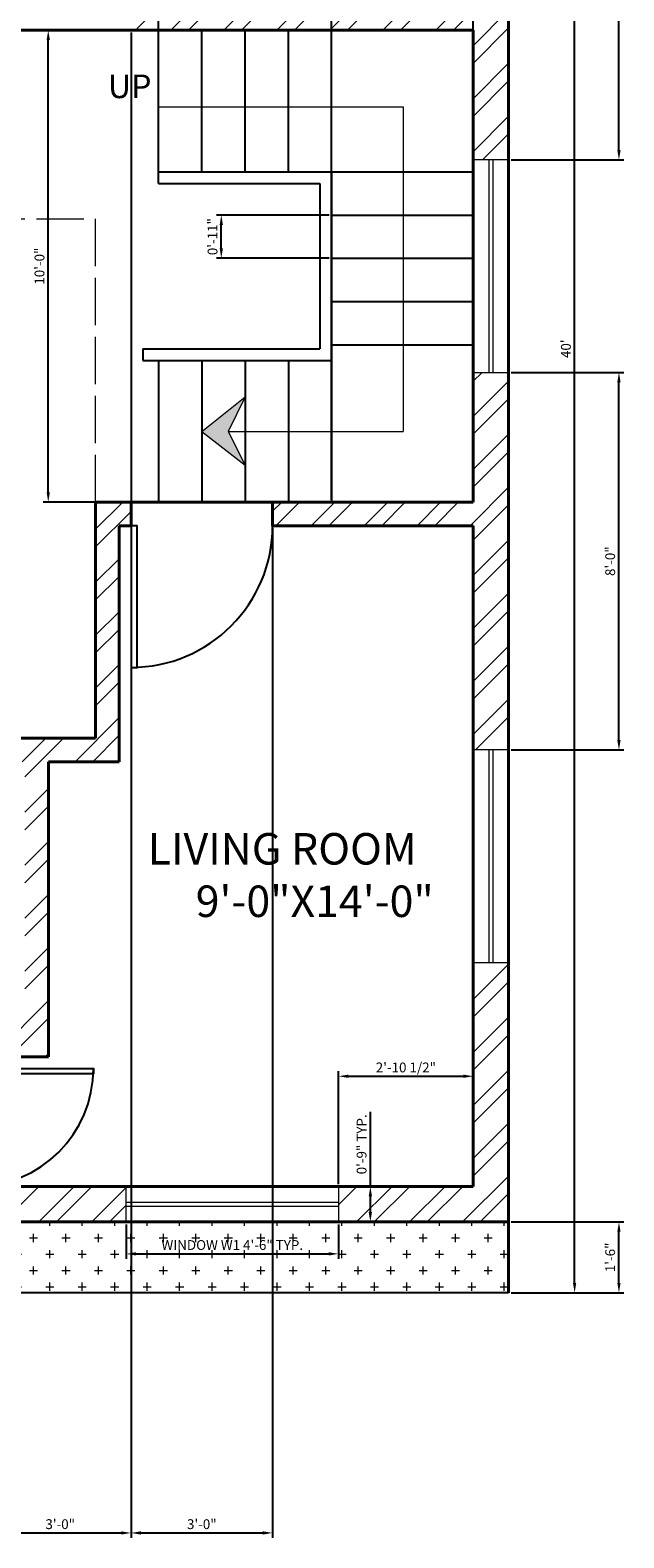
# Model space of a CAD drawing. Units: inches. Extents: x 201 to 622, y 55 to 632.
# Tile 2 of 3: x 471 to 622, y 56 to 439. Entities that reach past the tile are written whole.
import ezdxf

# ---------------------------------------------------------------- set-up
doc = ezdxf.new("R2010")
doc.units = ezdxf.units.IN
doc.linetypes.add('ACAD_ISO02W100', pattern=[15, 12, -3])
for name, color, linetype, lineweight in [('A-ANNO-DIMS', 2, 'Continuous', 18), ('A-ANNO-TEXT', 7, 'Continuous', 18), ('A-AREA-IDEN', 7, 'Continuous', 18), ('A-DOOR', 4, 'Continuous', 25), ('A-FLOR', 7, 'Continuous', 25), ('A-FLOR-OVHD', 7, 'ACAD_ISO02W100', 18), ('A-FLOR-STRS', 7, 'Continuous', 25), ('A-WALL', 7, 'Continuous', 40), ('A-WALL-PATT', 252, 'Continuous', 13)]:
    doc.layers.add(name, color=color, linetype=linetype, lineweight=lineweight)
for name, color, linetype, lineweight, true_color in [('A-ANNO-SYMB', 244, 'Continuous', 18, 0x991b1e), ('A-FLOR-PATT', 116, 'Continuous', 13, 0x136734), ('A-GLAZ', 152, 'Continuous', 18, 0x2776bb)]:
    doc.layers.add(name, color=color, linetype=linetype, lineweight=lineweight, true_color=true_color)
doc.styles.get("Standard").update_dxf_attribs({"font": 'arial.ttf'})
doc.dimstyles.new('ISO-25', dxfattribs={"dimtxt": 2.5, "dimasz": 2.5, "dimexe": 1.25, "dimexo": 0.625, "dimtad": 1, "dimlunit": 3, "dimtxsty": 'Standard', "dimcen": 2.5, "dimadec": 0, "dimazin": 0, "dimtfac": 1, "dimtmove": 0, "dimatfit": 3, "dimfxl": 1, "dimarcsym": 0})

# ---------------------------------------------------------------- blocks, each defined once
blk = doc.blocks.new('*U4')
for p, q in [((0, 0), (0, 6)), ((40, 0), (40, 6))]:
    blk.add_line(p, q)
blk.add_lwpolyline([(0, 0), (0, -40), (1.75, -40), (1.75, 0)], close=True)
blk.add_arc((0, 0), 40, 270, 360)
blk = doc.blocks.new('*U6')
for p, q in [((0, 0), (0, -6)), ((40, 0), (40, -6))]:
    blk.add_line(p, q)
blk.add_lwpolyline([(0, 0), (0, 40), (1.75, 40), (1.75, 0)], close=True)
blk.add_arc((0, 0), 40, 0, 90)
blk = doc.blocks.new('*D10')
at = {"layer": 'A-ANNO-DIMS', "color": 0, "lineweight": -2, "transparency": 16777216}
for p, q in [((592.99, 598.15), (610.4, 598.15)), ((609.15, 120.65), (609.15, 595.65)), ((592.99, 118.15), (610.4, 118.15))]:
    blk.add_line(p, q, dxfattribs=at)
at = {"layer": 'A-ANNO-DIMS', "color": 0, "transparency": 16777216}
for points in [[(608.73, 595.65), (609.56, 595.65), (609.15, 598.15)], [(608.73, 120.65), (609.56, 120.65), (609.15, 118.15)]]:
    blk.add_solid(points, dxfattribs=at)
at = {"layer": 'Defpoints', "color": 0, "transparency": 16777216}
for p in [(592.36, 598.15), (609.15, 598.15), (592.36, 118.15)]:
    blk.add_point(p, dxfattribs=at)
at = {"layer": 'A-ANNO-DIMS', "color": 0, "transparency": 16777216, "insert": (607.25, 358.15), "char_height": 2.5, "attachment_point": 5, "rotation": 90}
blk.add_mtext("40'", dxfattribs=at)
blk = doc.blocks.new('WIN-54')
for p, q in [((0, 5), (54, 5)), ((0, 4), (54, 4))]:
    blk.add_line(p, q)
blk.add_lwpolyline([(0, 9), (54, 9), (54, 0), (0, 0)], close=True)
blk = doc.blocks.new('WIN-54-B')
for p, q in [((0, 5), (54, 5)), ((0, 4), (54, 4))]:
    blk.add_line(p, q)
blk.add_lwpolyline([(0, 9), (54, 9), (54, 0), (0, 0)], close=True)
blk = doc.blocks.new('*D15')
at = {"layer": 'A-ANNO-DIMS', "color": 0, "lineweight": -2, "transparency": 16777216}
for p, q in [((495.11, 135.52), (495.11, 126.8)), ((549.11, 135.52), (549.11, 126.8)), ((497.61, 128.05), (546.61, 128.05))]:
    blk.add_line(p, q, dxfattribs=at)
at = {"layer": 'A-ANNO-DIMS', "color": 0, "transparency": 16777216}
for points in [[(497.61, 128.46), (497.61, 127.63), (495.11, 128.05)], [(546.61, 128.46), (546.61, 127.63), (549.11, 128.05)]]:
    blk.add_solid(points, dxfattribs=at)
at = {"layer": 'Defpoints', "color": 0, "transparency": 16777216}
for p in [(495.11, 136.15), (549.11, 136.15), (549.11, 128.05)]:
    blk.add_point(p, dxfattribs=at)
at = {"layer": 'A-ANNO-DIMS', "color": 0, "transparency": 16777216, "insert": (522.11, 129.97), "char_height": 2.5, "attachment_point": 5}
blk.add_mtext('WINDOW W1 4\'-6" TYP.', dxfattribs=at)
blk = doc.blocks.new('*D16')
at = {"layer": 'A-ANNO-DIMS', "color": 0, "lineweight": -2, "transparency": 16777216}
for p, q in [((557.21, 145.15), (557.21, 164.14)), ((549.73, 145.15), (558.46, 145.15)), ((557.21, 138.65), (557.21, 142.65)), ((549.73, 136.15), (558.46, 136.15))]:
    blk.add_line(p, q, dxfattribs=at)
at = {"layer": 'A-ANNO-DIMS', "color": 0, "transparency": 16777216}
for points in [[(556.79, 142.65), (557.63, 142.65), (557.21, 145.15)], [(556.79, 138.65), (557.63, 138.65), (557.21, 136.15)]]:
    blk.add_solid(points, dxfattribs=at)
at = {"layer": 'Defpoints', "color": 0, "transparency": 16777216}
for p in [(549.11, 145.15), (557.21, 145.15), (549.11, 136.15)]:
    blk.add_point(p, dxfattribs=at)
at = {"layer": 'A-ANNO-DIMS', "color": 0, "transparency": 16777216, "insert": (555.31, 155.89), "char_height": 2.5, "attachment_point": 5, "rotation": 90}
blk.add_mtext('0\'-9" TYP.', dxfattribs=at)
blk = doc.blocks.new('*D26')
at = {"layer": 'A-ANNO-DIMS', "color": 0, "lineweight": -2, "transparency": 16777216}
for p, q in [((547.36, 319.77), (547.36, 627.45)), ((549.86, 626.2), (580.86, 626.2)), ((583.36, 319.77), (583.36, 627.45))]:
    blk.add_line(p, q, dxfattribs=at)
at = {"layer": 'A-ANNO-DIMS', "color": 0, "transparency": 16777216}
for points in [[(549.86, 626.61), (549.86, 625.78), (547.36, 626.2)], [(580.86, 626.61), (580.86, 625.78), (583.36, 626.2)]]:
    blk.add_solid(points, dxfattribs=at)
at = {"layer": 'Defpoints', "color": 0, "transparency": 16777216}
for p in [(583.36, 626.2), (547.36, 319.15), (583.36, 319.15)]:
    blk.add_point(p, dxfattribs=at)
at = {"layer": 'A-ANNO-DIMS', "color": 0, "transparency": 16777216, "insert": (565.36, 628.1), "char_height": 2.5, "attachment_point": 5}
blk.add_mtext('3\'-0"', dxfattribs=at)
blk = doc.blocks.new('*D33')
at = {"layer": 'A-ANNO-DIMS', "color": 0, "lineweight": -2, "transparency": 16777216}
for p, q in [((592.99, 490.15), (621.66, 490.15)), ((620.41, 408.65), (620.41, 487.65)), ((592.99, 406.15), (621.66, 406.15))]:
    blk.add_line(p, q, dxfattribs=at)
at = {"layer": 'A-ANNO-DIMS', "color": 0, "transparency": 16777216}
for points in [[(620, 487.65), (620.83, 487.65), (620.41, 490.15)], [(620, 408.65), (620.83, 408.65), (620.41, 406.15)]]:
    blk.add_solid(points, dxfattribs=at)
at = {"layer": 'Defpoints', "color": 0, "transparency": 16777216}
for p in [(592.36, 490.15), (620.41, 490.15), (592.36, 406.15)]:
    blk.add_point(p, dxfattribs=at)
at = {"layer": 'A-ANNO-DIMS', "color": 0, "transparency": 16777216, "insert": (618.51, 448.15), "char_height": 2.5, "attachment_point": 5, "rotation": 90}
blk.add_mtext('7\'-0"', dxfattribs=at)
blk = doc.blocks.new('*D34')
at = {"layer": 'A-ANNO-DIMS', "color": 0, "lineweight": -2, "transparency": 16777216}
for p, q in [((592.99, 352.15), (621.66, 352.15)), ((620.41, 258.65), (620.41, 349.65)), ((592.99, 256.15), (621.66, 256.15))]:
    blk.add_line(p, q, dxfattribs=at)
at = {"layer": 'A-ANNO-DIMS', "color": 0, "transparency": 16777216}
for points in [[(620, 349.65), (620.83, 349.65), (620.41, 352.15)], [(620, 258.65), (620.83, 258.65), (620.41, 256.15)]]:
    blk.add_solid(points, dxfattribs=at)
at = {"layer": 'Defpoints', "color": 0, "transparency": 16777216}
for p in [(592.36, 352.15), (620.41, 352.15), (592.36, 256.15)]:
    blk.add_point(p, dxfattribs=at)
at = {"layer": 'A-ANNO-DIMS', "color": 0, "transparency": 16777216, "insert": (618.51, 304.15), "char_height": 2.5, "attachment_point": 5, "rotation": 90}
blk.add_mtext('8\'-0"', dxfattribs=at)
blk = doc.blocks.new('*D36')
at = {"layer": 'A-ANNO-DIMS', "color": 0, "lineweight": -2, "transparency": 16777216}
for p, q in [((549.11, 145.77), (549.11, 174.45)), ((551.61, 173.2), (580.86, 173.2)), ((583.36, 145.77), (583.36, 174.45))]:
    blk.add_line(p, q, dxfattribs=at)
at = {"layer": 'A-ANNO-DIMS', "color": 0, "transparency": 16777216}
for points in [[(551.61, 173.61), (551.61, 172.78), (549.11, 173.2)], [(580.86, 173.61), (580.86, 172.78), (583.36, 173.2)]]:
    blk.add_solid(points, dxfattribs=at)
at = {"layer": 'Defpoints', "color": 0, "transparency": 16777216}
for p in [(583.36, 173.2), (549.11, 145.15), (583.36, 145.15)]:
    blk.add_point(p, dxfattribs=at)
at = {"layer": 'A-ANNO-DIMS', "color": 0, "transparency": 16777216, "insert": (566.24, 175.11), "char_height": 2.5, "attachment_point": 5}
blk.add_mtext('2\'-10 1/2"', dxfattribs=at)
blk = doc.blocks.new('*D41')
at = {"layer": 'A-ANNO-DIMS', "color": 0, "lineweight": -2, "transparency": 16777216}
for p, q in [((546.74, 392.15), (518.06, 392.15)), ((519.31, 383.65), (519.31, 389.65)), ((546.74, 381.15), (518.06, 381.15))]:
    blk.add_line(p, q, dxfattribs=at)
at = {"layer": 'A-ANNO-DIMS', "color": 0, "transparency": 16777216}
for points in [[(518.9, 389.65), (519.73, 389.65), (519.31, 392.15)], [(518.9, 383.65), (519.73, 383.65), (519.31, 381.15)]]:
    blk.add_solid(points, dxfattribs=at)
at = {"layer": 'Defpoints', "color": 0, "transparency": 16777216}
for p in [(519.31, 392.15), (547.36, 392.15), (547.36, 381.15)]:
    blk.add_point(p, dxfattribs=at)
at = {"layer": 'A-ANNO-DIMS', "color": 0, "transparency": 16777216, "insert": (517.41, 386.65), "char_height": 2.5, "attachment_point": 5, "rotation": 90}
blk.add_mtext('0\'-11"', dxfattribs=at)
blk = doc.blocks.new('*D43')
at = {"layer": 'A-ANNO-DIMS', "color": 0, "lineweight": -2, "transparency": 16777216}
for p, q in [((592.99, 136.15), (621.66, 136.15)), ((620.41, 120.65), (620.41, 133.65)), ((592.99, 118.15), (621.66, 118.15))]:
    blk.add_line(p, q, dxfattribs=at)
at = {"layer": 'A-ANNO-DIMS', "color": 0, "transparency": 16777216}
for points in [[(620, 133.65), (620.83, 133.65), (620.41, 136.15)], [(620, 120.65), (620.83, 120.65), (620.41, 118.15)]]:
    blk.add_solid(points, dxfattribs=at)
at = {"layer": 'Defpoints', "color": 0, "transparency": 16777216}
for p in [(592.36, 136.15), (620.41, 136.15), (592.36, 118.15)]:
    blk.add_point(p, dxfattribs=at)
at = {"layer": 'A-ANNO-DIMS', "color": 0, "transparency": 16777216, "insert": (618.51, 127.15), "char_height": 2.5, "attachment_point": 5, "rotation": 90}
blk.add_mtext('1\'-6"', dxfattribs=at)
blk = doc.blocks.new('*D46')
at = {"layer": 'A-ANNO-DIMS', "color": 0, "lineweight": -2, "transparency": 16777216}
for p, q in [((502.74, 439.15), (474.06, 439.15)), ((475.31, 321.65), (475.31, 436.65)), ((502.74, 319.15), (474.06, 319.15))]:
    blk.add_line(p, q, dxfattribs=at)
at = {"layer": 'A-ANNO-DIMS', "color": 0, "transparency": 16777216}
for points in [[(474.9, 436.65), (475.73, 436.65), (475.31, 439.15)], [(474.9, 321.65), (475.73, 321.65), (475.31, 319.15)]]:
    blk.add_solid(points, dxfattribs=at)
at = {"layer": 'Defpoints', "color": 0, "transparency": 16777216}
for p in [(475.31, 439.15), (503.36, 439.15), (503.36, 319.15)]:
    blk.add_point(p, dxfattribs=at)
at = {"layer": 'A-ANNO-DIMS', "color": 0, "transparency": 16777216, "insert": (473.41, 379.15), "char_height": 2.5, "attachment_point": 5, "rotation": 90}
blk.add_mtext('10\'-0"', dxfattribs=at)
blk = doc.blocks.new('*D49')
at = {"layer": 'A-ANNO-DIMS', "color": 0, "lineweight": -2, "transparency": 16777216}
for p, q in [((460.36, 438.52), (460.36, 55.85)), ((496.36, 438.52), (496.36, 55.85)), ((462.86, 57.1), (493.86, 57.1))]:
    blk.add_line(p, q, dxfattribs=at)
at = {"layer": 'A-ANNO-DIMS', "color": 0, "transparency": 16777216}
for points in [[(462.86, 57.51), (462.86, 56.68), (460.36, 57.1)], [(493.86, 57.51), (493.86, 56.68), (496.36, 57.1)]]:
    blk.add_solid(points, dxfattribs=at)
at = {"layer": 'Defpoints', "color": 0, "transparency": 16777216}
for p in [(460.36, 439.15), (496.36, 439.15), (496.36, 57.1)]:
    blk.add_point(p, dxfattribs=at)
at = {"layer": 'A-ANNO-DIMS', "color": 0, "transparency": 16777216, "insert": (478.36, 59), "char_height": 2.5, "attachment_point": 5}
blk.add_mtext('3\'-0"', dxfattribs=at)
blk = doc.blocks.new('*D54')
at = {"layer": 'A-ANNO-DIMS', "color": 0, "lineweight": -2, "transparency": 16777216}
for p, q in [((496.36, 312.52), (496.36, 55.85)), ((532.36, 312.52), (532.36, 55.85)), ((498.86, 57.1), (529.86, 57.1))]:
    blk.add_line(p, q, dxfattribs=at)
at = {"layer": 'A-ANNO-DIMS', "color": 0, "transparency": 16777216}
for points in [[(498.86, 57.51), (498.86, 56.68), (496.36, 57.1)], [(529.86, 57.51), (529.86, 56.68), (532.36, 57.1)]]:
    blk.add_solid(points, dxfattribs=at)
at = {"layer": 'Defpoints', "color": 0, "transparency": 16777216}
for p in [(496.36, 313.15), (532.36, 313.15), (532.36, 57.1)]:
    blk.add_point(p, dxfattribs=at)
at = {"layer": 'A-ANNO-DIMS', "color": 0, "transparency": 16777216, "insert": (514.36, 59), "char_height": 2.5, "attachment_point": 5}
blk.add_mtext('3\'-0"', dxfattribs=at)
blk = doc.blocks.new('*D55')
at = {"layer": 'A-ANNO-DIMS', "color": 0, "lineweight": -2, "transparency": 16777216}
for p, q in [((503.36, 403.77), (503.36, 627.45)), ((505.86, 626.2), (580.86, 626.2)), ((583.36, 403.77), (583.36, 627.45))]:
    blk.add_line(p, q, dxfattribs=at)
at = {"layer": 'A-ANNO-DIMS', "color": 0, "transparency": 16777216}
for points in [[(505.86, 626.61), (505.86, 625.78), (503.36, 626.2)], [(580.86, 626.61), (580.86, 625.78), (583.36, 626.2)]]:
    blk.add_solid(points, dxfattribs=at)
at = {"layer": 'Defpoints', "color": 0, "transparency": 16777216}
for p in [(583.36, 626.2), (503.36, 403.15), (583.36, 403.15)]:
    blk.add_point(p, dxfattribs=at)
at = {"layer": 'A-ANNO-DIMS', "color": 0, "transparency": 16777216, "insert": (543.36, 628.1), "char_height": 2.5, "attachment_point": 5}
blk.add_mtext('6\'-8"', dxfattribs=at)

msp = doc.modelspace()

# ---------------------------------------------------------------- hatches: boundary and pattern name
at = {"layer": 'A-ANNO-SYMB'}
h = msp.add_hatch(color=256, dxfattribs=at)
h.dxf.hatch_style = 1
h.paths.add_polyline_path([(525.362, 345.885), (514.362, 337.147), (525.362, 328.593), (521.099, 337.147)])
at = {"layer": 'A-FLOR-PATT'}
h = msp.add_hatch(dxfattribs=at)
h.set_pattern_fill('CROSS', color=256, scale=0.65)
h.paths.add_polyline_path([(592.362, 136.147), (451.858, 136.147), (451.858, 118.147), (592.362, 118.147)])
at = {"layer": 'A-WALL-PATT'}
h = msp.add_hatch(dxfattribs=at)
h.set_pattern_fill('ANSI32', color=256)
h.paths.add_polyline_path([(241.362, 589.147), (286.362, 589.147), (286.362, 598.147), (232.362, 598.147), (232.362, 418.002), (241.362, 418.002), (241.362, 439.147), (337.362, 439.147), (337.362, 436.147), (343.362, 436.147), (343.362, 439.147), (346.362, 439.147), (346.362, 445.147), (241.362, 445.147)])
h.paths.add_polyline_path([(394.362, 493.147), (391.362, 493.147), (391.362, 589.147), (426.354, 589.147), (426.354, 598.147), (340.362, 598.147), (340.362, 589.147), (385.362, 589.147), (385.362, 445.147), (382.362, 445.147), (382.362, 439.147), (391.362, 439.147), (391.362, 487.147), (394.362, 487.147)])
h.paths.add_polyline_path([(457.362, 589.147), (493.362, 589.147), (493.362, 598.147), (447.354, 598.147), (447.354, 589.147), (451.362, 589.147), (451.362, 493.147), (424.362, 493.147), (424.362, 487.147), (451.362, 487.147), (451.362, 439.147), (460.362, 439.147), (460.362, 445.147), (457.362, 445.147)])
h.paths.add_polyline_path([(592.362, 598.147), (547.362, 598.147), (547.362, 589.147), (550.362, 589.147), (583.362, 589.147), (583.362, 544.147), (592.362, 544.147)])
h.paths.add_polyline_path([(592.362, 490.147), (583.362, 490.147), (583.362, 445.147), (496.362, 445.147), (496.362, 439.147), (583.362, 439.147), (583.362, 406.147), (592.362, 406.147)])
h.paths.add_polyline_path([(592.362, 352.147), (583.362, 352.147), (583.362, 319.147), (532.362, 319.147), (532.362, 313.147), (583.362, 313.147), (583.362, 256.147), (592.362, 256.147)])
h.paths.add_polyline_path([(592.362, 202.147), (583.362, 202.147), (583.362, 145.147), (549.11, 145.147), (549.11, 136.147), (592.362, 136.147)])
h.paths.add_polyline_path([(493.362, 313.147), (496.362, 313.147), (496.362, 319.147), (487.362, 319.147), (487.362, 259.147), (409.362, 259.147), (409.362, 250.147), (415.362, 250.147), (415.362, 253.147), (469.362, 253.147), (469.362, 187.147), (448.415, 187.147), (448.415, 178.147), (451.858, 178.147), (451.858, 175.147), (457.858, 175.147), (457.858, 178.147), (475.362, 178.147), (475.362, 253.147), (493.362, 253.147)])
h.paths.add_polyline_path([(495.11, 145.147), (457.858, 145.147), (451.858, 145.147), (451.858, 136.147), (495.11, 136.147)])
h.paths.add_polyline_path([(367.362, 178.147), (370.362, 178.147), (370.362, 183.547), (370.362, 187.147), (367.362, 187.147), (367.362, 220.147), (361.362, 220.147), (361.362, 127.147), (326.862, 127.147), (326.862, 118.147), (367.362, 118.147)])
h.paths.add_polyline_path([(272.862, 127.147), (241.362, 127.147), (241.362, 259.147), (361.362, 259.147), (361.362, 256.147), (361.962, 256.147), (367.362, 256.147), (367.362, 289.147), (361.362, 289.147), (361.362, 265.147), (241.362, 265.147), (241.362, 385.147), (361.362, 385.147), (361.362, 361.147), (367.362, 361.147), (367.362, 391.147), (343.362, 391.147), (343.362, 406.147), (338.862, 406.147), (337.362, 406.147), (337.362, 391.147), (241.362, 391.147), (241.362, 397.002), (232.362, 397.002), (232.362, 118.147), (272.862, 118.147)])
h.paths.add_polyline_path([(417.381, 187.147), (415.362, 187.147), (415.362, 220.147), (410.862, 220.147), (409.362, 220.147), (409.362, 187.147), (406.181, 187.147, -0.0250471), (406.362, 183.547), (406.362, 178.147), (417.381, 178.147)])

# ---------------------------------------------------------------- linework, layer by layer
at = {"layer": 'A-ANNO-SYMB'}
for p, q in [((503.362, 419.647), (565.547, 419.647)), ((565.547, 419.647), (565.547, 337.147)), ((514.362, 337.147), (525.362, 345.885)), ((525.362, 345.885), (521.099, 337.147)), ((514.362, 337.147), (525.362, 328.593)), ((521.099, 337.147), (565.547, 337.147)), ((521.099, 337.147), (525.362, 328.593))]:
    msp.add_line(p, q, dxfattribs=at)
at = {"layer": 'A-FLOR'}
msp.add_line((592.362, 118.147), (367.362, 118.147), dxfattribs=at)
at = {"layer": 'A-FLOR-OVHD'}
for p in [(367.362, 391.147), (487.362, 319.147)]:
    msp.add_line(p, (487.362, 391.147), dxfattribs=at)
at = {"layer": 'A-FLOR-STRS'}
for p, q in [((503.362, 400.147), (503.362, 439.147)), ((514.362, 403.147), (514.362, 439.147)), ((525.362, 403.147), (525.362, 439.147)), ((536.362, 403.147), (536.362, 439.147)), ((547.362, 403.147), (547.362, 439.147)), ((503.362, 403.147), (547.362, 403.147)), ((547.362, 403.147), (547.362, 355.147)), ((547.362, 403.147), (583.362, 403.147)), ((503.362, 400.147), (544.362, 400.147)), ((544.362, 400.147), (544.362, 358.147)), ((547.362, 392.147), (583.362, 392.147)), ((547.362, 381.147), (583.362, 381.147)), ((547.362, 370.147), (583.362, 370.147)), ((499.362, 358.147), (544.362, 358.147)), ((499.362, 358.147), (499.362, 355.147)), ((547.362, 359.147), (583.362, 359.147)), ((499.362, 355.147), (547.362, 355.147)), ((503.362, 355.147), (503.362, 319.147)), ((514.362, 355.147), (514.362, 319.147)), ((525.362, 355.147), (525.362, 319.147)), ((536.362, 355.147), (536.362, 319.147)), ((547.362, 355.147), (547.362, 319.147))]:
    msp.add_line(p, q, dxfattribs=at)
at = {"layer": 'A-WALL'}
for p, q in [((592.362, 598.147), (592.362, 118.147)), ((451.362, 439.147), (583.362, 439.147)), ((583.362, 439.147), (583.362, 319.147)), ((487.362, 319.147), (583.362, 319.147)), ((487.362, 259.147), (487.362, 319.147)), ((496.362, 313.147), (496.362, 319.147)), ((532.362, 313.147), (532.362, 319.147)), ((493.362, 313.147), (496.362, 313.147)), ((493.362, 253.147), (493.362, 313.147)), ((532.362, 313.147), (583.362, 313.147)), ((583.362, 313.147), (583.362, 145.147)), ((409.362, 259.147), (487.362, 259.147)), ((475.362, 178.147), (475.362, 253.147)), ((475.362, 253.147), (493.362, 253.147)), ((457.858, 178.147), (475.362, 178.147)), ((457.858, 145.147), (583.362, 145.147)), ((451.858, 136.147), (592.362, 136.147))]:
    msp.add_line(p, q, dxfattribs=at)

# ---------------------------------------------------------------- block references
at = {"layer": 'A-DOOR', "xscale": 0.9, "yscale": 0.9, "zscale": 0.9}
msp.add_blockref('*U4', (496.362, 313.147), dxfattribs=at)
at = {"layer": 'A-DOOR', "xscale": 0.75, "yscale": 0.75, "zscale": 0.75, "rotation": 270}
msp.add_blockref('*U6', (456.779, 175.147), dxfattribs=at)
at = {"layer": 'A-GLAZ', "extrusion": (0, 0, -1), "zscale": -1, "rotation": 270}
for name, p in [('WIN-54', (-592.362, 406.147)), ('WIN-54-B', (-592.362, 256.147))]:
    msp.add_blockref(name, p, dxfattribs=at)
at = {"layer": 'A-GLAZ'}
msp.add_blockref('WIN-54', (495.11, 136.147), dxfattribs=at)

# ---------------------------------------------------------------- texts
at = {"layer": 'A-ANNO-TEXT', "insert": (490.477, 427.872), "char_height": 6, "attachment_point": 1}
msp.add_mtext_dynamic_manual_height_columns('UP', width=12.88452, gutter_width=12.5, heights=[0], dxfattribs=at)
at = {"layer": 'A-AREA-IDEN', "insert": (500.581, 235.023), "char_height": 8, "attachment_point": 1}
msp.add_mtext_dynamic_manual_height_columns('LIVING ROOM        9\'-0"X14\'-0"', width=74.40783, gutter_width=12.5, heights=[0], dxfattribs=at)

# ---------------------------------------------------------------- dimensions: what is measured, and where the dimension line sits
at = {"layer": 'A-ANNO-DIMS'}
for base, p1, p2, picture, middle in [((583.362, 626.197), (503.362, 403.147), (583.362, 403.147), '*D55', (543.362, 628.099)), ((583.362, 626.197), (547.362, 319.147), (583.362, 319.147), '*D26', (565.362, 628.1)), ((496.362, 57.097), (460.362, 439.147), (496.362, 439.147), '*D49', (478.362, 59)), ((532.362, 57.097), (496.362, 313.147), (532.362, 313.147), '*D54', (514.362, 59)), ((583.362, 173.197), (549.11, 145.147), (583.362, 145.147), '*D36', (566.236, 175.115))]:
    dim = msp.add_linear_dim(base=base, p1=p1, p2=p2, dimstyle='ISO-25', override={"dimdec": 1, "dimlfac": 1, "dimrnd": 0, "dimzin": 1, "dimdsep": 46, "dimlunit": 4, "dimfrac": 2}, dxfattribs=at)
    dim.commit()
    dim.dimension.update_dxf_attribs({"geometry": picture, "text_midpoint": middle})
for base, p1, p2, override, picture, middle in [((609.147, 598.147), (592.362, 118.147), (592.362, 598.147), {"dimclrd": 0, "dimclre": 0, "dimclrt": 0}, '*D10', (607.246, 358.147)), ((620.412, 490.147), (592.362, 406.147), (592.362, 490.147), {"dimdec": 1, "dimlfac": 1, "dimrnd": 0, "dimzin": 1, "dimdsep": 46, "dimlunit": 4, "dimfrac": 2}, '*D33', (618.51, 448.147)), ((475.312, 439.147), (503.362, 319.147), (503.362, 439.147), {"dimdec": 1, "dimlfac": 1, "dimrnd": 0, "dimzin": 1, "dimdsep": 46, "dimlunit": 4, "dimfrac": 2}, '*D46', (473.41, 379.147)), ((519.312, 392.147), (547.362, 381.147), (547.362, 392.147), {"dimdec": 1, "dimlfac": 1, "dimrnd": 0, "dimzin": 1, "dimdsep": 46, "dimlunit": 4, "dimfrac": 2}, '*D41', (517.41, 386.647)), ((620.412, 352.147), (592.362, 256.147), (592.362, 352.147), {"dimdec": 1, "dimlfac": 1, "dimrnd": 0, "dimzin": 1, "dimdsep": 46, "dimlunit": 4, "dimfrac": 2}, '*D34', (618.51, 304.147)), ((620.412, 136.147), (592.362, 118.147), (592.362, 136.147), {"dimdec": 1, "dimlfac": 1, "dimrnd": 0, "dimzin": 1, "dimdsep": 46, "dimlunit": 4, "dimfrac": 2}, '*D43', (618.51, 127.147))]:
    dim = msp.add_linear_dim(base=base, p1=p1, p2=p2, angle=90, dimstyle='ISO-25', override=override, dxfattribs=at)
    dim.commit()
    dim.dimension.update_dxf_attribs({"geometry": picture, "text_midpoint": middle})
dim = msp.add_linear_dim(base=(557.21, 145.147), p1=(549.11, 136.147), p2=(549.11, 145.147), angle=90, text='<> TYP.', dimstyle='ISO-25', override={"dimdec": 1, "dimlfac": 1, "dimrnd": 0, "dimzin": 1, "dimdsep": 46, "dimlunit": 4, "dimfrac": 2}, dxfattribs=at)
dim.commit()
dim.dimension.update_dxf_attribs({"geometry": '*D16', "text_midpoint": (555.308, 155.892)})
dim = msp.add_linear_dim(base=(549.11, 128.047), p1=(495.11, 136.147), p2=(549.11, 136.147), text='WINDOW W1 <> TYP.', dimstyle='ISO-25', override={"dimdec": 1, "dimlfac": 1, "dimrnd": 0, "dimzin": 1, "dimdsep": 46, "dimlunit": 4, "dimfrac": 2}, dxfattribs=at)
dim.commit()
dim.dimension.update_dxf_attribs({"geometry": '*D15', "text_midpoint": (522.11, 129.966)})

doc.saveas('drawing.dxf')
